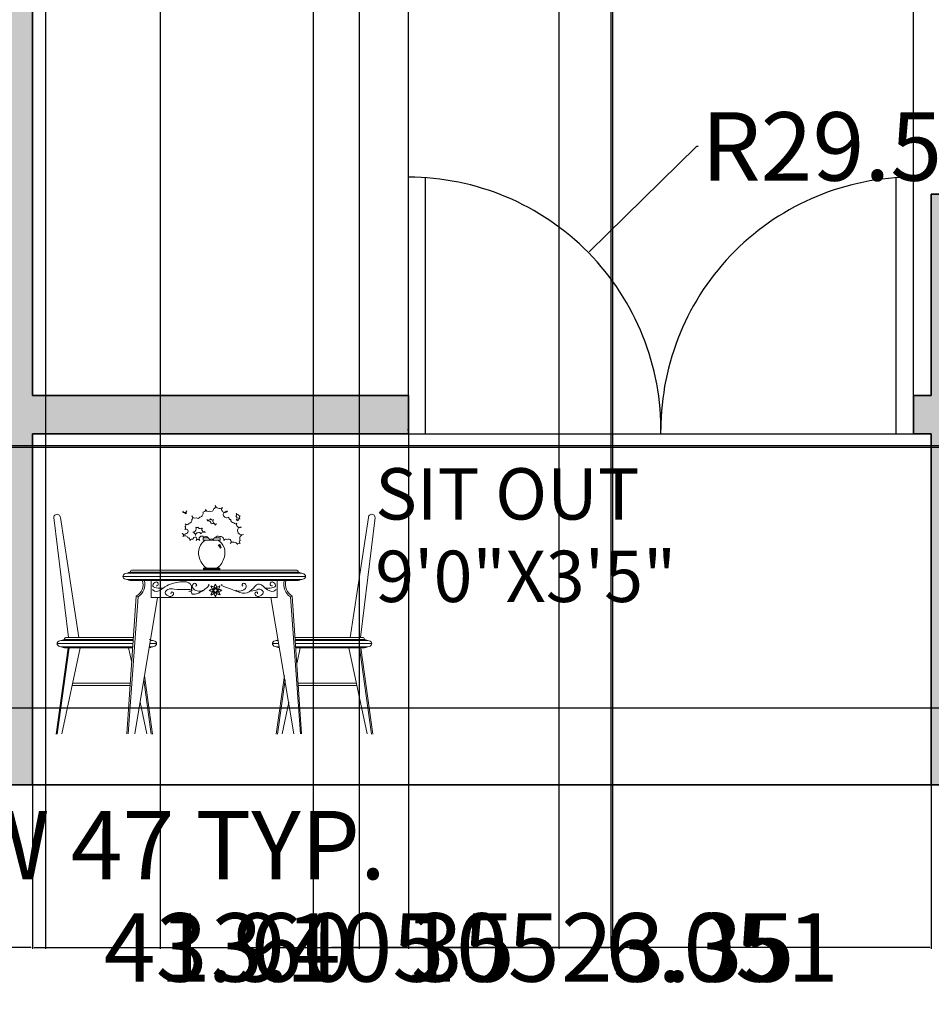
# Model space of a CAD drawing. Units: inches. Extents: x -24 to 368, y -370 to 58.
# Tile 3 of 9: x 130 to 237, y -370 to -255. Entities that reach past the tile are written whole.
import ezdxf

# ---------------------------------------------------------------- set-up
doc = ezdxf.new("R2010")
doc.units = ezdxf.units.IN
doc.header["$MEASUREMENT"] = 0
for name, color, linetype, lineweight in [('A-ANNO-DIMS', 2, 'Continuous', 18), ('A-AREA-IDEN', 7, 'Continuous', 18), ('A-WALL', 7, 'Continuous', 35), ('Furniture', 7, 'Continuous', 15)]:
    doc.layers.add(name, color=color, linetype=linetype, lineweight=lineweight)
doc.layers.add('A-DOOR', color=40, linetype='Continuous', lineweight=25, true_color=0xf8d731)
doc.layers.add('A-WALL-PATT', color=18, linetype='Continuous', lineweight=13, true_color=0x000000)
doc.styles.get("Standard").update_dxf_attribs({"font": 'arial.ttf'})
doc.dimstyles.get("Standard").update_dxf_attribs({"dimtxt": 8, "dimasz": 0.18, "dimexe": 0.18, "dimexo": 0.0625, "dimgap": 0.09, "dimtad": 0, "dimtih": 1, "dimtoh": 1, "dimdec": 4, "dimzin": 0, "dimdsep": 46, "dimlunit": 3, "dimtxsty": 'Standard', "dimcen": 0.09, "dimclre": 5, "dimclrt": 6, "dimadec": 0, "dimazin": 0, "dimtfac": 1, "dimtdec": 4, "dimtofl": 0, "dimtmove": 0, "dimatfit": 3, "dimfxl": 1, "dimtolj": 1, "dimtzin": 0, "dimarcsym": 0})

# ---------------------------------------------------------------- blocks, each defined once
blk = doc.blocks.new('*D15')
at = {"layer": 'A-ANNO-DIMS', "color": 5, "lineweight": -2, "transparency": 16777216}
for p, q in [((37.41, -344.42), (37.41, -351.59)), ((84.41, -344.42), (84.41, -351.59))]:
    blk.add_line(p, q, dxfattribs=at)
at = {"layer": 'A-ANNO-DIMS', "color": 0, "lineweight": -2, "transparency": 16777216}
for p, q in [((37.59, -351.41), (84.23, -351.41)), ((84.41, -351.41), (84.59, -351.41))]:
    blk.add_line(p, q, dxfattribs=at)
at = {"layer": 'A-ANNO-DIMS', "color": 0, "transparency": 16777216}
for points in [[(37.59, -351.38), (37.59, -351.44), (37.41, -351.41)], [(84.23, -351.38), (84.23, -351.44), (84.41, -351.41)]]:
    blk.add_solid(points, dxfattribs=at)
at = {"layer": 'Defpoints', "color": 0, "transparency": 16777216}
for p in [(37.41, -344.36), (84.41, -344.36), (84.41, -351.41)]:
    blk.add_point(p, dxfattribs=at)
at = {"layer": 'A-ANNO-DIMS', "color": 6, "transparency": 16777216, "insert": (130.38, -351.41), "char_height": 8, "attachment_point": 5}
blk.add_mtext('\\A1;WINDOW 47 TYP.', dxfattribs=at)
blk = doc.blocks.new('*D28')
at = {"layer": 'A-ANNO-DIMS', "color": 5, "lineweight": -2, "transparency": 16777216}
for p, q in [((84.41, -344.42), (84.41, -363.55)), ((131.66, -344.42), (131.66, -363.55))]:
    blk.add_line(p, q, dxfattribs=at)
at = {"layer": 'A-ANNO-DIMS', "color": 0, "lineweight": -2, "transparency": 16777216}
for p, q in [((84.59, -363.37), (94.29, -363.37)), ((131.48, -363.37), (121.78, -363.37))]:
    blk.add_line(p, q, dxfattribs=at)
at = {"layer": 'A-ANNO-DIMS', "color": 0, "transparency": 16777216}
for points in [[(84.59, -363.34), (84.59, -363.4), (84.41, -363.37)], [(131.48, -363.34), (131.48, -363.4), (131.66, -363.37)]]:
    blk.add_solid(points, dxfattribs=at)
at = {"layer": 'Defpoints', "color": 0, "transparency": 16777216}
for p in [(84.41, -344.36), (131.66, -344.36), (131.66, -363.37)]:
    blk.add_point(p, dxfattribs=at)
at = {"layer": 'A-ANNO-DIMS', "color": 6, "transparency": 16777216, "insert": (108.03, -363.37), "char_height": 8, "attachment_point": 5}
blk.add_mtext('\\A1;47.26', dxfattribs=at)
blk = doc.blocks.new('*D29')
at = {"layer": 'A-ANNO-DIMS', "color": 5, "lineweight": -2, "transparency": 16777216}
for p, q in [((131.66, -344.42), (131.66, -363.55)), ((236.66, -344.42), (236.66, -363.55))]:
    blk.add_line(p, q, dxfattribs=at)
at = {"layer": 'A-ANNO-DIMS', "color": 0, "lineweight": -2, "transparency": 16777216}
for p, q in [((131.84, -363.37), (175.58, -363.37)), ((236.48, -363.37), (192.74, -363.37))]:
    blk.add_line(p, q, dxfattribs=at)
at = {"layer": 'A-ANNO-DIMS', "color": 0, "transparency": 16777216}
for points in [[(131.84, -363.34), (131.84, -363.4), (131.66, -363.37)], [(236.48, -363.34), (236.48, -363.4), (236.66, -363.37)]]:
    blk.add_solid(points, dxfattribs=at)
at = {"layer": 'Defpoints', "color": 0, "transparency": 16777216}
for p in [(131.66, -344.36), (236.66, -344.36), (236.66, -363.37)]:
    blk.add_point(p, dxfattribs=at)
at = {"layer": 'A-ANNO-DIMS', "color": 6, "transparency": 16777216, "insert": (184.16, -363.37), "char_height": 8, "attachment_point": 5}
blk.add_mtext('\\A1;105', dxfattribs=at)
blk = doc.blocks.new('*D42')
at = {"layer": 'A-ANNO-DIMS', "color": 5, "lineweight": -2, "transparency": 16777216}
for p, q in [((169.81, 24.59), (169.81, -363.55)), ((193.16, 24.58), (193.16, -363.55))]:
    blk.add_line(p, q, dxfattribs=at)
at = {"layer": 'A-ANNO-DIMS', "color": 0, "lineweight": -2, "transparency": 16777216}
for p, q in [((169.99, -363.37), (192.98, -363.37)), ((193.16, -363.37), (193.34, -363.37))]:
    blk.add_line(p, q, dxfattribs=at)
at = {"layer": 'A-ANNO-DIMS', "color": 0, "transparency": 16777216}
for points in [[(169.99, -363.34), (169.99, -363.4), (169.81, -363.37)], [(192.98, -363.34), (192.98, -363.4), (193.16, -363.37)]]:
    blk.add_solid(points, dxfattribs=at)
at = {"layer": 'Defpoints', "color": 0, "transparency": 16777216}
for p in [(169.81, 24.65), (193.16, 24.64), (193.16, -363.37)]:
    blk.add_point(p, dxfattribs=at)
at = {"layer": 'A-ANNO-DIMS', "color": 6, "transparency": 16777216, "insert": (207.03, -363.37), "char_height": 8, "attachment_point": 5}
blk.add_mtext('\\A1;23.35', dxfattribs=at)
blk = doc.blocks.new('*D46')
at = {"layer": 'A-ANNO-DIMS', "color": 5, "lineweight": -2, "transparency": 16777216}
for p, q in [((13.22, -304.91), (341.36, -304.91)), ((13.22, -335.36), (341.36, -335.36))]:
    blk.add_line(p, q, dxfattribs=at)
at = {"layer": 'A-ANNO-DIMS', "color": 0, "lineweight": -2, "transparency": 16777216}
for p, q in [((341.18, -305.09), (341.18, -315.95)), ((341.18, -335.18), (341.18, -324.31))]:
    blk.add_line(p, q, dxfattribs=at)
at = {"layer": 'A-ANNO-DIMS', "color": 0, "transparency": 16777216}
for points in [[(341.15, -305.09), (341.21, -305.09), (341.18, -304.91)], [(341.15, -335.18), (341.21, -335.18), (341.18, -335.36)]]:
    blk.add_solid(points, dxfattribs=at)
at = {"layer": 'Defpoints', "color": 0, "transparency": 16777216}
for p in [(13.16, -304.91), (341.18, -304.91), (13.16, -335.36)]:
    blk.add_point(p, dxfattribs=at)
at = {"layer": 'A-ANNO-DIMS', "color": 6, "transparency": 16777216, "insert": (341.18, -320.13), "char_height": 8, "attachment_point": 5}
blk.add_mtext('\\A1;30.45', dxfattribs=at)
blk = doc.blocks.new('*D51')
at = {"layer": 'A-ANNO-DIMS', "color": 5, "lineweight": -2, "transparency": 16777216}
for p, q in [((175.57, -303.29), (175.57, 52.85)), ((234.57, -303.29), (234.57, 52.85))]:
    blk.add_line(p, q, dxfattribs=at)
at = {"layer": 'A-ANNO-DIMS', "color": 0, "lineweight": -2, "transparency": 16777216}
for p, q in [((175.75, 52.67), (199.24, 52.67)), ((234.39, 52.67), (210.9, 52.67))]:
    blk.add_line(p, q, dxfattribs=at)
at = {"layer": 'A-ANNO-DIMS', "color": 0, "transparency": 16777216}
for points in [[(175.75, 52.7), (175.75, 52.64), (175.57, 52.67)], [(234.39, 52.7), (234.39, 52.64), (234.57, 52.67)]]:
    blk.add_solid(points, dxfattribs=at)
at = {"layer": 'Defpoints', "color": 0, "transparency": 16777216}
for p in [(234.57, 52.67), (175.57, -303.36), (234.57, -303.36)]:
    blk.add_point(p, dxfattribs=at)
at = {"layer": 'A-ANNO-DIMS', "color": 6, "transparency": 16777216, "insert": (205.07, 52.67), "char_height": 8, "attachment_point": 5}
blk.add_mtext('\\A1;59', dxfattribs=at)
blk = doc.blocks.new('*D52')
at = {"layer": 'A-ANNO-DIMS', "color": 5, "lineweight": -2, "transparency": 16777216}
for p, q in [((131.66, -303.42), (131.66, -363.55)), ((175.57, -303.42), (175.57, -363.55))]:
    blk.add_line(p, q, dxfattribs=at)
at = {"layer": 'A-ANNO-DIMS', "color": 0, "lineweight": -2, "transparency": 16777216}
for p, q in [((131.84, -363.37), (140.64, -363.37)), ((175.39, -363.37), (166.59, -363.37))]:
    blk.add_line(p, q, dxfattribs=at)
at = {"layer": 'A-ANNO-DIMS', "color": 0, "transparency": 16777216}
for points in [[(131.84, -363.34), (131.84, -363.4), (131.66, -363.37)], [(175.39, -363.34), (175.39, -363.4), (175.57, -363.37)]]:
    blk.add_solid(points, dxfattribs=at)
at = {"layer": 'Defpoints', "color": 0, "transparency": 16777216}
for p in [(131.66, -303.36), (175.57, -303.36), (175.57, -363.37)]:
    blk.add_point(p, dxfattribs=at)
at = {"layer": 'A-ANNO-DIMS', "color": 6, "transparency": 16777216, "insert": (153.62, -363.37), "char_height": 8, "attachment_point": 5}
blk.add_mtext('\\A1;43.91', dxfattribs=at)
blk = doc.blocks.new('*D56')
at = {"layer": 'A-ANNO-DIMS', "color": 5, "lineweight": -2, "transparency": 16777216}
for p, q in [((164.43, -152.42), (164.43, -363.55)), ((199.43, -152.42), (199.43, -363.55))]:
    blk.add_line(p, q, dxfattribs=at)
at = {"layer": 'A-ANNO-DIMS', "color": 0, "lineweight": -2, "transparency": 16777216}
for p, q in [((164.61, -363.37), (176.08, -363.37)), ((199.25, -363.37), (187.78, -363.37))]:
    blk.add_line(p, q, dxfattribs=at)
at = {"layer": 'A-ANNO-DIMS', "color": 0, "transparency": 16777216}
for points in [[(164.61, -363.34), (164.61, -363.4), (164.43, -363.37)], [(199.25, -363.34), (199.25, -363.4), (199.43, -363.37)]]:
    blk.add_solid(points, dxfattribs=at)
at = {"layer": 'Defpoints', "color": 0, "transparency": 16777216}
for p in [(164.43, -152.36), (199.43, -152.36), (199.43, -363.37)]:
    blk.add_point(p, dxfattribs=at)
at = {"layer": 'A-ANNO-DIMS', "color": 6, "transparency": 16777216, "insert": (181.93, -363.37), "char_height": 8, "attachment_point": 5}
blk.add_mtext('\\A1;35', dxfattribs=at)
blk = doc.blocks.new('*D58')
at = {"layer": 'A-ANNO-DIMS', "color": 5, "lineweight": -2, "transparency": 16777216}
for p, q in [((133.16, -31.92), (133.16, -363.55)), ((146.57, -31.92), (146.57, -363.55))]:
    blk.add_line(p, q, dxfattribs=at)
at = {"layer": 'A-ANNO-DIMS', "color": 0, "lineweight": -2, "transparency": 16777216}
for p, q in [((133.34, -363.37), (146.39, -363.37)), ((146.57, -363.37), (146.75, -363.37))]:
    blk.add_line(p, q, dxfattribs=at)
at = {"layer": 'A-ANNO-DIMS', "color": 0, "transparency": 16777216}
for points in [[(133.34, -363.34), (133.34, -363.4), (133.16, -363.37)], [(146.39, -363.34), (146.39, -363.4), (146.57, -363.37)]]:
    blk.add_solid(points, dxfattribs=at)
at = {"layer": 'Defpoints', "color": 0, "transparency": 16777216}
for p in [(133.16, -31.86), (146.57, -31.86), (146.57, -363.37)]:
    blk.add_point(p, dxfattribs=at)
at = {"layer": 'A-ANNO-DIMS', "color": 6, "transparency": 16777216, "insert": (163.1, -363.37), "char_height": 8, "attachment_point": 5}
blk.add_mtext('\\A1;13.405', dxfattribs=at)
blk = doc.blocks.new('*D60')
at = {"layer": 'A-ANNO-DIMS', "color": 5, "lineweight": -2, "transparency": 16777216}
for p, q in [((133.16, -93.92), (133.16, -363.55)), ((193.16, -95.92), (193.16, -363.55))]:
    blk.add_line(p, q, dxfattribs=at)
at = {"layer": 'A-ANNO-DIMS', "color": 0, "lineweight": -2, "transparency": 16777216}
for p, q in [((133.34, -363.37), (157.33, -363.37)), ((192.98, -363.37), (168.99, -363.37))]:
    blk.add_line(p, q, dxfattribs=at)
at = {"layer": 'A-ANNO-DIMS', "color": 0, "transparency": 16777216}
for points in [[(133.34, -363.34), (133.34, -363.4), (133.16, -363.37)], [(192.98, -363.34), (192.98, -363.4), (193.16, -363.37)]]:
    blk.add_solid(points, dxfattribs=at)
at = {"layer": 'Defpoints', "color": 0, "transparency": 16777216}
for p in [(133.16, -93.86), (193.16, -95.86), (193.16, -363.37)]:
    blk.add_point(p, dxfattribs=at)
at = {"layer": 'A-ANNO-DIMS', "color": 6, "transparency": 16777216, "insert": (163.16, -363.37), "char_height": 8, "attachment_point": 5}
blk.add_mtext('\\A1;60', dxfattribs=at)
blk = doc.blocks.new('*D64')
at = {"layer": 'A-ANNO-DIMS', "color": 5, "lineweight": -2, "transparency": 16777216}
for p, q in [((105.73, -304.73), (341.36, -304.73)), ((106.02, -335.36), (341.36, -335.36))]:
    blk.add_line(p, q, dxfattribs=at)
at = {"layer": 'A-ANNO-DIMS', "color": 0, "lineweight": -2, "transparency": 16777216}
for p, q in [((341.18, -304.91), (341.18, -315.86)), ((341.18, -335.18), (341.18, -324.22))]:
    blk.add_line(p, q, dxfattribs=at)
at = {"layer": 'A-ANNO-DIMS', "color": 0, "transparency": 16777216}
for points in [[(341.15, -304.91), (341.21, -304.91), (341.18, -304.73)], [(341.15, -335.18), (341.21, -335.18), (341.18, -335.36)]]:
    blk.add_solid(points, dxfattribs=at)
at = {"layer": 'Defpoints', "color": 0, "transparency": 16777216}
for p in [(105.67, -304.73), (341.18, -304.73), (105.95, -335.36)]:
    blk.add_point(p, dxfattribs=at)
at = {"layer": 'A-ANNO-DIMS', "color": 6, "transparency": 16777216, "insert": (341.18, -320.04), "char_height": 8, "attachment_point": 5}
blk.add_mtext('\\A1;30.63', dxfattribs=at)
blk = doc.blocks.new('*D65')
at = {"layer": 'A-ANNO-DIMS', "color": 5, "lineweight": -2, "transparency": 16777216}
for p, q in [((105.95, -335.29), (105.95, 52.85)), ((127.16, -335.29), (127.16, 52.85))]:
    blk.add_line(p, q, dxfattribs=at)
at = {"layer": 'A-ANNO-DIMS', "color": 0, "lineweight": -2, "transparency": 16777216}
for p, q in [((106.13, 52.67), (126.98, 52.67)), ((127.16, 52.67), (127.34, 52.67))]:
    blk.add_line(p, q, dxfattribs=at)
at = {"layer": 'A-ANNO-DIMS', "color": 0, "transparency": 16777216}
for points in [[(106.13, 52.7), (106.13, 52.64), (105.95, 52.67)], [(126.98, 52.7), (126.98, 52.64), (127.16, 52.67)]]:
    blk.add_solid(points, dxfattribs=at)
at = {"layer": 'Defpoints', "color": 0, "transparency": 16777216}
for p in [(127.16, 52.67), (105.95, -335.36), (127.16, -335.36)]:
    blk.add_point(p, dxfattribs=at)
at = {"layer": 'A-ANNO-DIMS', "color": 6, "transparency": 16777216, "insert": (140.23, 52.67), "char_height": 8, "attachment_point": 5}
blk.add_mtext('\\A1;21.21', dxfattribs=at)
blk = doc.blocks.new('*D70')
at = {"layer": 'A-ANNO-DIMS', "color": 5, "lineweight": -2, "transparency": 16777216}
for p, q in [((193.16, -95.92), (193.16, -363.55)), ((199.21, -95.92), (199.21, -363.55))]:
    blk.add_line(p, q, dxfattribs=at)
at = {"layer": 'A-ANNO-DIMS', "color": 0, "lineweight": -2, "transparency": 16777216}
for p, q in [((193.34, -363.37), (199.03, -363.37)), ((199.21, -363.37), (199.39, -363.37))]:
    blk.add_line(p, q, dxfattribs=at)
at = {"layer": 'A-ANNO-DIMS', "color": 0, "transparency": 16777216}
for points in [[(193.34, -363.34), (193.34, -363.4), (193.16, -363.37)], [(199.03, -363.34), (199.03, -363.4), (199.21, -363.37)]]:
    blk.add_solid(points, dxfattribs=at)
at = {"layer": 'Defpoints', "color": 0, "transparency": 16777216}
for p in [(193.16, -95.86), (199.21, -95.86), (199.21, -363.37)]:
    blk.add_point(p, dxfattribs=at)
at = {"layer": 'A-ANNO-DIMS', "color": 6, "transparency": 16777216, "insert": (212.23, -363.37), "char_height": 8, "attachment_point": 5}
blk.add_mtext('\\A1;6.051', dxfattribs=at)
blk = doc.blocks.new('*D71')
at = {"layer": 'A-ANNO-DIMS', "color": 0, "lineweight": -2, "transparency": 16777216}
for p, q in [((209.23, -269.76), (196.73, -282.05)), ((209.41, -269.76), (209.23, -269.76))]:
    blk.add_line(p, q, dxfattribs=at)
at = {"layer": 'A-ANNO-DIMS', "color": 5, "lineweight": -2, "transparency": 16777216}
for p, q in [((175.48, -302.86), (175.66, -302.86)), ((175.57, -302.95), (175.57, -302.77))]:
    blk.add_line(p, q, dxfattribs=at)
at = {"layer": 'A-ANNO-DIMS', "color": 0, "transparency": 16777216}
blk.add_solid([(196.71, -282.03), (196.76, -282.07), (196.61, -282.17)], dxfattribs=at)
at = {"layer": 'Defpoints', "color": 0, "transparency": 16777216}
for p in [(196.61, -282.17), (175.57, -302.86)]:
    blk.add_point(p, dxfattribs=at)
at = {"layer": 'A-ANNO-DIMS', "color": 6, "transparency": 16777216, "insert": (229.92, -269.76), "char_height": 8, "attachment_point": 5}
blk.add_mtext('\\A1;R29.504', dxfattribs=at)

msp = doc.modelspace()

# ---------------------------------------------------------------- hatches: boundary and pattern name
at = {"layer": 'A-WALL-PATT'}
h = msp.add_hatch(color=256, dxfattribs=at)
h.dxf.hatch_style = 1
h.paths.add_polyline_path([(13.1621, -93.8573), (80.4499, -93.8573), (80.4499, -89.3573), (13.1621, -89.3573), (13.1621, -61.0987), (4.1621, -61.0987), (4.1621, -149.8573), (13.1621, -149.8573)])
h.paths.add_polyline_path([(146.5668, -27.3573), (133.1621, -27.3573), (133.1621, 10.3323), (133.1272, 10.3313), (133.1621, 24.6427), (139.8141, 24.6427), (139.8141, 33.6427), (95.3329, 33.6427), (95.3329, 24.6427), (128.6621, 24.6427), (128.6621, -89.3573), (127.4499, -89.3573), (127.4499, -93.8573), (133.1621, -93.8573), (133.1621, -31.8573), (146.5668, -31.8573)])
h.paths.add_polyline_path([(197.6621, 24.6427), (236.2134, 24.6427), (236.2134, 33.6427), (169.8141, 33.6427), (169.8141, 24.6427), (193.1621, 24.6427), (193.1621, -27.3573), (181.5668, -27.3573), (181.5668, -31.8573), (193.1621, -31.8573), (193.1621, -95.8573), (199.2127, -95.8573), (199.2127, -91.3573), (197.6621, -91.3573)])
h.paths.add_polyline_path([(322.1621, -52.531), (313.1621, -52.531), (313.1621, -91.3573), (246.2127, -91.3573), (246.2127, -95.8573), (246.6621, -95.8573), (246.6621, -104.9077), (251.1621, -104.9077), (251.1621, -95.8573), (313.1621, -95.8573), (313.1621, -105.6922), (317.6621, -105.6922), (322.1621, -105.6922)])
h.paths.add_polyline_path([(322.1621, -135.6922), (313.1621, -135.6922), (313.1621, -147.8573), (251.1621, -147.8573), (251.1621, -139.9077), (246.6621, -139.9077), (246.6621, -147.8573), (199.43, -147.8573), (199.43, -152.3573), (313.1621, -152.3573), (313.1621, -194.6142), (317.6621, -194.6142), (322.1621, -194.6142)])
h.paths.add_polyline_path([(322.1621, -241.6142), (313.1621, -241.6142), (313.1621, -275.3573), (287.3912, -275.3573), (287.3912, -279.8573), (313.1621, -279.8573), (313.1621, -335.3573), (298.077, -335.3573), (298.077, -344.3573), (322.1621, -344.3573)])
h.paths.add_polyline_path([(263.077, -335.3573), (241.1621, -335.3573), (241.1621, -279.8573), (252.3912, -279.8573), (252.3912, -275.3573), (236.6621, -275.3573), (236.6621, -298.8573), (234.5689, -298.8573), (234.5689, -303.3573), (236.6621, -303.3573), (236.6621, -344.3573), (263.077, -344.3573), (263.077, -339.8573)])
h.paths.add_polyline_path([(175.5689, -298.8573), (131.6621, -298.8573), (131.6621, -152.3573), (164.43, -152.3573), (164.43, -147.8573), (127.1621, -147.8573), (127.1621, -232.8573), (117.1621, -232.8573), (117.1621, -237.3573), (127.1621, -237.3573), (127.1621, -335.3573), (84.4055, -335.3573), (84.4055, -344.3573), (131.6621, -344.3573), (131.6621, -303.3573), (175.5689, -303.3573)])
h.paths.add_polyline_path([(70.1621, -232.8573), (13.1621, -232.8573), (13.1621, -196.8573), (4.1621, -196.8573), (4.1621, -257.9061), (13.1621, -257.9061), (13.1621, -237.3573), (70.1621, -237.3573)])
h.paths.add_polyline_path([(13.1621, -304.9061), (4.1621, -304.9061), (4.1621, -344.3573), (37.4055, -344.3573), (37.4055, -335.3573), (13.1621, -335.3573)])
h.paths.add_polyline_path([(322.1621, 33.6427), (283.2134, 33.6427), (283.2134, 24.6427), (313.1621, 24.6427), (313.1621, 11.9273), (313.4656, 11.629), (313.1621, 11.629), (313.1621, -5.531), (322.1621, -5.531)])
h.paths.add_polyline_path([(48.3329, 33.6427), (4.1621, 33.6427), (4.1621, -14.0987), (13.1621, -14.0987), (13.1621, 24.6427), (48.3329, 24.6427)])

# ---------------------------------------------------------------- linework, layer by layer
at = {"layer": 'A-DOOR'}
for p, q in [((175.5689, -303.3573), (175.5689, -273.3573)), ((177.5689, -303.3573), (177.5689, -273.3573)), ((232.5689, -303.3573), (232.5689, -273.3573)), ((234.5689, -303.3573), (234.5689, -273.3573)), ((175.5689, -298.8573), (175.5689, -303.3573)), ((234.5689, -298.8573), (234.5689, -303.3573)), ((175.5689, -303.3573), (234.5689, -303.3573))]:
    msp.add_line(p, q, dxfattribs=at)
for centre, radius, start, end in [((175.5689, -302.8615), 29.5042, 359.037068, 90), ((234.5689, -302.8531), 29.4958, 90, 180.016185)]:
    msp.add_arc(centre, radius, start, end, dxfattribs=at)
at = {"layer": 'A-WALL'}
for p, q in [((131.6621, -298.8573), (131.6621, -152.3573)), ((236.6621, -275.3573), (236.6621, -298.8573)), ((252.3912, -275.3573), (236.6621, -275.3573)), ((175.5689, -298.8573), (131.6621, -298.8573)), ((236.6621, -298.8573), (234.5689, -298.8573)), ((131.6621, -344.3573), (131.6621, -303.3573)), ((175.5689, -303.3573), (131.6621, -303.3573)), ((236.6621, -303.3573), (234.5689, -303.3573)), ((236.6621, -303.3573), (236.6621, -344.3573)), ((322.1621, -344.3573), (4.1621, -344.3573))]:
    msp.add_line(p, q, dxfattribs=at)
at = {"layer": 'Furniture'}
for p, q in [((135.8503, -327.1311), (134.1515, -313.1372)), ((137.0665, -327.1311), (134.918, -313.1372)), ((168.7647, -327.1311), (170.9132, -313.1372)), ((169.9809, -327.1311), (171.6798, -313.1372)), ((151.5962, -315.7681), (151.5962, -315.4901)), ((152.1996, -315.4901), (151.5962, -315.4901)), ((153.5975, -315.7681), (151.5962, -315.7681)), ((153.5975, -315.4901), (153.0416, -315.4901)), ((153.4992, -316.2761), (153.3679, -316.3866)), ((153.5975, -315.7681), (153.5975, -315.4901)), ((153.7066, -316.5869), (153.5753, -316.6974)), ((162.9698, -319.6366), (142.8068, -319.6366)), ((162.706, -319.5137), (143.0694, -319.5137)), ((162.4915, -319.268), (143.3397, -319.268)), ((151.6287, -319.0514), (151.6287, -319.3097)), ((153.547, -319.0514), (151.6287, -319.0514)), ((153.547, -319.1126), (151.6287, -319.1126)), ((153.547, -319.1839), (151.6287, -319.1839)), ((153.547, -319.0514), (153.547, -319.3097)), ((163.5544, -320.0051), (142.2221, -320.0051)), ((162.9698, -320.3737), (142.8068, -320.3737)), ((162.7065, -320.4966), (143.0694, -320.4966)), ((145.5371, -322.4623), (145.5371, -320.4966)), ((160.2388, -322.4623), (160.2388, -320.4966)), ((152.6166, -321.2765), (152.6067, -321.2468)), ((152.6415, -321.2599), (152.6071, -321.2467)), ((152.6415, -321.2599), (152.617, -321.2764)), ((152.6626, -321.9067), (152.6683, -321.8759)), ((152.6924, -321.9041), (152.663, -321.9066)), ((152.6924, -321.9041), (152.6687, -321.8758)), ((153.0833, -321.5062), (153.089, -321.4754)), ((153.113, -321.5036), (153.0837, -321.5061)), ((153.113, -321.5036), (153.0893, -321.4753)), ((153.1491, -321.7914), (153.1392, -321.7617)), ((153.1681, -321.7725), (153.1396, -321.7616)), ((153.3229, -321.2371), (153.3149, -321.2132)), ((153.3477, -321.2205), (153.3221, -321.2107)), ((153.3477, -321.2205), (153.3233, -321.237)), ((153.3676, -321.8451), (153.3723, -321.8194)), ((153.3973, -321.8424), (153.368, -321.8449)), ((153.3973, -321.8424), (153.377, -321.8181)), ((153.4425, -321.5935), (153.4325, -321.5638)), ((153.4673, -321.5769), (153.4329, -321.5637)), ((153.4673, -321.5769), (153.4429, -321.5934)), ((143.7643, -322.3142), (142.6946, -338.4264)), ((143.9893, -322.4112), (142.8252, -338.4264)), ((146.2743, -322.4623), (143.5955, -338.4264)), ((143.9847, -322.4143), (143.7643, -322.3142)), ((160.2388, -322.4623), (145.5371, -322.4623)), ((152.9505, -322.2262), (152.9526, -322.2148)), ((152.9767, -322.2429), (152.953, -322.2146)), ((152.9767, -322.2429), (152.9604, -322.2443)), ((159.5016, -322.4623), (162.1803, -338.4264)), ((161.7866, -322.4112), (162.9506, -338.4264)), ((161.7911, -322.4143), (162.0115, -322.3142)), ((162.0115, -322.3142), (163.0813, -338.4264)), ((134.531, -327.8682), (143.3956, -327.8682)), ((143.42, -327.4996), (135.1157, -327.4996)), ((143.4282, -327.3768), (135.3794, -327.3768)), ((143.4445, -327.1311), (135.6486, -327.1311)), ((145.3672, -327.8682), (146.1532, -327.8682)), ((145.5686, -327.4996), (145.429, -327.4996)), ((145.9549, -327.8682), (146.1532, -327.8682)), ((159.8763, -327.8682), (159.678, -327.8682)), ((160.4087, -327.8682), (159.678, -327.8682)), ((160.2626, -327.4996), (160.3468, -327.4996)), ((162.3867, -327.1311), (170.1826, -327.1311)), ((162.403, -327.3768), (170.4518, -327.3768)), ((162.4112, -327.4996), (170.7155, -327.4996)), ((171.3002, -327.8682), (162.4357, -327.8682)), ((135.808, -328.3597), (134.4065, -338.4343)), ((135.9595, -328.3597), (134.558, -338.4343)), ((143.3709, -328.2397), (135.0546, -328.2397)), ((137.2121, -328.3597), (135.0878, -338.4264)), ((143.3629, -328.3597), (135.3783, -328.3597)), ((142.8844, -328.3597), (143.2484, -330.0847)), ((145.6297, -328.2397), (145.3048, -328.2397)), ((160.2016, -328.2397), (160.471, -328.2397)), ((162.4603, -328.2397), (170.7766, -328.2397)), ((162.4683, -328.3597), (170.4529, -328.3597)), ((162.9469, -328.3597), (162.5828, -330.0847)), ((168.6191, -328.3597), (170.7434, -338.4264)), ((169.8717, -328.3597), (171.2732, -338.4343)), ((170.0232, -328.3597), (171.4248, -338.4343)), ((143.0881, -332.4987), (136.3387, -332.4987)), ((144.6572, -332.0992), (145.5385, -338.4343)), ((144.7401, -331.6055), (145.6901, -338.4343)), ((161.0912, -331.6055), (160.1412, -338.4343)), ((161.174, -332.0992), (160.2927, -338.4343)), ((162.7431, -332.4987), (169.4925, -332.4987)), ((143.0718, -332.7444), (136.3664, -332.7444)), ((162.7594, -332.7444), (169.5444, -332.7444)), ((144.2215, -334.6959), (145.0087, -338.4264)), ((161.6097, -334.6959), (160.8225, -338.4264))]:
    msp.add_line(p, q, dxfattribs=at)
for centre, radius, start, end in [((152.7358, -311.842), 0.2969, 286.313852, 32.574057), ((153.5211, -311.498), 0.5659, 198.991201, 305.251406), ((134.5347, -313.1313), 0.3833, 359.123141, 180.876859), ((149.3969, -312.3909), 0.1639, 184.864514, 291.124719), ((149.1815, -312.4743), 0.0869, 306.869898, 53.130102), ((149.3101, -312.7314), 0.2026, 5.906141, 112.166346), ((149.4942, -312.3632), 0.1847, 258.055823, 4.316028), ((149.6263, -312.7314), 0.1165, 63.434949, 169.695154), ((149.7826, -312.4882), 0.1737, 126.869898, 233.130102), ((150.5956, -312.8565), 0.3422, 192.907409, 299.167613), ((150.0953, -313.1553), 0.278, 306.869898, 53.130102), ((151.1689, -312.6446), 0.4291, 275.110418, 21.370622), ((151.6067, -312.2207), 0.2702, 261.869898, 8.130102), ((152.1799, -312.1269), 0.3108, 190.304846, 296.565051), ((152.4648, -312.0783), 0.3577, 245.924502, 352.184706), ((154.0144, -312.1825), 0.278, 126.869898, 233.130102), ((154.1395, -312.186), 0.3648, 216.869898, 323.130102), ((154.348, -312.8148), 0.4184, 78.503437, 184.763642), ((154.348, -312.7106), 0.4395, 198.434949, 304.695154), ((155.3173, -312.7592), 0.1942, 296.565051, 42.825256), ((155.2444, -313.204), 0.3146, 313.210089, 59.470294), ((155.6231, -312.6133), 0.1639, 184.864514, 291.124719), ((155.8559, -312.7662), 0.1737, 180, 286.260205), ((155.9288, -313.0233), 0.0936, 105.068488, 211.328693), ((171.2965, -313.1313), 0.3833, 359.123141, 180.876859), ((149.3692, -314.01), 0.1942, 296.565051, 42.825256), ((149.7027, -313.6695), 0.2828, 227.489553, 333.749758), ((149.9529, -313.4715), 0.3231, 270.61606, 16.876265), ((150.9535, -312.9468), 0.2828, 227.489553, 333.749758), ((152.2043, -313.1692), 0.2828, 227.489553, 333.749758), ((152.0027, -313.4784), 0.1013, 337.833654, 84.093859), ((152.1834, -313.8641), 0.3581, 357.776039, 104.036243), ((152.5586, -313.2839), 0.1013, 185.906141, 292.166346), ((152.7393, -314.1351), 0.3245, 21.345787, 127.605991), ((152.708, -313.2943), 0.139, 216.869898, 323.130102), ((152.9547, -313.5583), 0.2258, 126.869898, 233.130102), ((153.0659, -313.6626), 0.2583, 197.216074, 303.476278), ((153.1771, -314.01), 0.1357, 76.675469, 182.935673), ((154.824, -313.1414), 0.2363, 162.897271, 269.157476), ((155.1367, -313.4228), 0.3194, 171.869898, 278.130102), ((155.3833, -313.6313), 0.2285, 208.123735, 314.38394), ((155.5397, -313.5583), 0.1484, 16.313852, 122.574057), ((155.7308, -313.9579), 0.2487, 138.964655, 245.224859), ((155.8072, -313.4367), 0.1484, 106.313852, 212.574057), ((155.835, -313.3464), 0.0869, 36.869898, 143.130102), ((155.9601, -313.1623), 0.1433, 140.906141, 247.166346), ((149.3726, -314.823), 0.278, 216.869898, 323.130102), ((149.0565, -315.2017), 0.2318, 319.864514, 66.124719), ((149.4734, -315.6395), 0.375, 23.4774, 129.737605), ((149.3205, -314.3644), 0.2258, 306.869898, 53.130102), ((149.6158, -314.7084), 0.2285, 28.123735, 134.38394), ((149.5602, -314.7118), 0.2801, 277.125016, 23.385221), ((150.4462, -314.5069), 0.3194, 261.869898, 8.130102), ((150.408, -314.9585), 0.1357, 346.675469, 92.935673), ((150.54, -315.1635), 0.1737, 343.739795, 90), ((150.9604, -315.1635), 0.2583, 84.596209, 190.856413), ((150.8458, -314.1351), 0.1737, 216.869898, 323.130102), ((150.6512, -314.3714), 0.1433, 320.906141, 67.166346), ((151.2175, -314.1733), 0.242, 195.832387, 302.092591), ((151.1133, -315.1114), 0.242, 15.832387, 122.092591), ((151.4295, -314.3158), 0.1042, 216.869898, 323.130102), ((151.6935, -315.1322), 0.3581, 59.703552, 165.963757), ((151.6275, -314.5312), 0.1911, 126.869898, 233.130102), ((151.7456, -314.618), 0.242, 195.832387, 302.092591), ((156.0157, -314.6285), 0.3931, 81.869898, 188.130102), ((155.8697, -314.0448), 0.2801, 209.744881, 316.005086), ((156.1269, -314.6563), 0.5011, 183.17983, 289.440035), ((156.3492, -315.6082), 0.4827, 96.61346, 202.873665), ((149.8139, -315.7264), 0.2363, 342.897271, 89.157476), ((150.2517, -315.8897), 0.2318, 49.864514, 156.124719), ((150.6964, -315.6951), 0.2958, 77.106256, 183.366461), ((150.6165, -315.6013), 0.2432, 306.869898, 53.130102), ((150.9847, -315.9626), 0.278, 36.869898, 143.130102), ((152.7694, -317.2379), 1.721, 121.342885, 197.015329), ((151.353, -315.6013), 0.2432, 126.869898, 233.130102), ((151.4295, -315.5735), 0.278, 36.869898, 143.130102), ((151.8707, -315.8098), 0.4586, 12.246333, 118.506538), ((152.5378, -315.9418), 0.317, 27.407575, 133.66778), ((153.0451, -315.7264), 0.2363, 90.842524, 197.102729), ((153.3161, -315.5874), 0.2912, 54.223922, 160.484127), ((152.4244, -317.2379), 1.721, 342.984671, 58.657115), ((152.8803, -316.9365), 0.735, 18.989745, 48.438613), ((152.9564, -316.8744), 0.735, 18.989745, 48.438613), ((153.5836, -315.7715), 0.4315, 356.76899, 103.029195), ((153.0117, -316.826), 0.735, 18.989745, 48.438613), ((154.2264, -315.8897), 0.2318, 49.864514, 156.124719), ((154.5669, -315.9209), 0.2828, 26.250242, 132.510447), ((154.6433, -315.9453), 0.2318, 293.875281, 40.135486), ((155.1297, -316.5602), 0.5626, 27.989238, 134.249443), ((155.8176, -316.3309), 0.1942, 63.434949, 169.695154), ((156.04, -315.9765), 0.2258, 126.869898, 233.130102), ((153.473, -317.1425), 2.4244, 194.303833, 231.032589), ((151.7208, -317.1425), 2.4244, 308.967411, 345.696167), ((142.4924, -320.0051), 0.2703, 133.570645, 226.429355), ((142.7457, -320.2714), 0.6377, 84.502825, 133.570645), ((143.0677, -319.8521), 0.3384, 89.708291, 140.434352), ((143.3397, -319.5383), 0.2703, 90, 174.784091), ((162.4368, -319.5383), 0.2703, 5.215909, 90), ((162.7089, -319.8521), 0.3384, 39.565648, 90.291709), ((163.0309, -320.2714), 0.6377, 46.429355, 95.497175), ((163.2841, -320.0051), 0.2703, 313.570645, 46.429355), ((142.7457, -319.7389), 0.6377, 226.429355, 275.497175), ((143.0677, -320.1581), 0.3384, 219.565648, 270.291709), ((142.9967, -320.9382), 1.5756, 299.155129, 16.277185), ((142.9967, -320.9382), 1.7762, 303.796641, 13.185856), ((154.0039, -321.6566), 1.1976, 142.485612, 217.514388), ((154.5523, -321.6346), 1.714, 154.818742, 205.181258), ((152.0514, -321.6346), 1.1976, 322.485612, 37.514388), ((151.5029, -321.6566), 1.714, 334.818742, 25.181258), ((162.7792, -320.9382), 1.7762, 166.814144, 236.203359), ((162.7792, -320.9382), 1.5756, 163.722815, 240.844871), ((162.7089, -320.1581), 0.3384, 269.708291, 320.434352), ((163.0309, -319.7389), 0.6377, 264.502825, 313.570645), ((153.0166, -322.6218), 1.1976, 52.485612, 127.514388), ((153.0166, -320.1208), 1.714, 244.818742, 295.181258), ((153.0386, -323.1703), 1.714, 64.818742, 115.181258), ((153.0386, -320.6693), 1.1976, 232.485612, 307.514388), ((154.098, -320.5596), 1.714, 199.818742, 250.181258), ((152.3295, -322.3281), 1.1976, 7.485612, 82.514388), ((154.1135, -322.7159), 1.714, 109.818742, 160.181258), ((152.3451, -320.9475), 1.1976, 277.485612, 352.514388), ((153.7101, -322.3436), 1.1976, 97.485612, 172.514388), ((151.9417, -320.5752), 1.714, 289.818742, 340.181258), ((153.7257, -320.963), 1.1976, 187.485612, 262.514388), ((151.9572, -322.7315), 1.714, 19.818742, 70.181258), ((134.8013, -327.8682), 0.2703, 133.570645, 226.429355), ((135.0546, -328.1344), 0.6377, 84.502825, 133.570645), ((135.3766, -327.7152), 0.3384, 89.708291, 140.434352), ((135.6486, -327.4014), 0.2703, 90, 174.784091), ((145.3077, -327.7152), 0.3384, 39.565648, 90.291709), ((145.6297, -328.1344), 0.6377, 46.429355, 95.497175), ((145.8829, -327.8682), 0.2703, 313.570645, 46.429355), ((159.9483, -327.8682), 0.2703, 133.570645, 226.429355), ((160.2016, -328.1344), 0.6377, 84.502825, 133.570645), ((160.5235, -327.7152), 0.3384, 123.700532, 140.434352), ((170.1826, -327.4014), 0.2703, 5.215909, 90), ((170.4546, -327.7152), 0.3384, 39.565648, 90.291709), ((170.7766, -328.1344), 0.6377, 46.429355, 95.497175), ((171.0299, -327.8682), 0.2703, 313.570645, 46.429355), ((135.0546, -327.602), 0.6377, 226.429355, 275.497175), ((135.3766, -328.0212), 0.3384, 219.565648, 270.291709), ((145.3077, -328.0212), 0.3384, 269.708291, 320.434352), ((145.6297, -327.602), 0.6377, 264.502825, 313.570645), ((160.2016, -327.602), 0.6377, 226.429355, 275.497175), ((160.5235, -328.0212), 0.3384, 219.565648, 264.461782), ((170.4546, -328.0212), 0.3384, 269.708291, 320.434352), ((170.7766, -327.602), 0.6377, 264.502825, 313.570645)]:
    msp.add_arc(centre, radius, start, end, dxfattribs=at)
for points, knots in [([(152.1721, -320.9715), (152.5148, -320.9428), (151.3046, -322.017), (149.9846, -322.3116), (150.5997, -320.3243), (148.0352, -320.6728), (146.9584, -321.3253), (146.1071, -321.9472), (145.7472, -321.6139), (145.6615, -321.5344)], [0, 0, 0, 0, 1.03178829, 2.30706702, 3.06879509, 5.53273575, 6.51138896, 7.57049354, 7.90185408, 7.90185408, 7.90185408, 7.90185408]), ([(146.8549, -321.3689), (146.7013, -321.374), (146.3404, -321.386), (145.5428, -321.2831), (145.8581, -320.6993), (146.3074, -320.5846), (146.4015, -321.1158), (146.1697, -321.1069), (146.0924, -321.104)], [0, 0, 0, 0, 0.49725443, 1.16840045, 1.6574062, 1.92466762, 2.32749044, 2.52912891, 2.52912891, 2.52912891, 2.52912891]), ([(151.4759, -321.6338), (151.7266, -321.797), (150.369, -321.8033), (150.2154, -320.9354), (150.7204, -320.7418), (150.88, -321.0635), (150.754, -321.1192), (150.7135, -321.1371)], [0, 0, 0, 0, 0.89750365, 1.58014669, 1.88576066, 2.13797138, 2.25745142, 2.25745142, 2.25745142, 2.25745142]), ([(153.8305, -320.9715), (153.2296, -320.9212), (155.6018, -321.7901), (156.713, -322.1598), (157.4601, -321.3743), (158.1301, -320.6857), (158.8562, -321.437), (159.6662, -321.9397), (160.0281, -321.6124), (160.1144, -321.5344)], [0, 0, 0, 0, 1.80901962, 3.08429834, 4.28493376, 4.71080628, 5.6894595, 6.74856407, 7.07992461, 7.07992461, 7.07992461, 7.07992461]), ([(155.4714, -321.6338), (155.2207, -321.797), (156.5783, -321.8033), (156.7319, -320.9354), (156.2269, -320.7418), (156.0673, -321.0635), (156.1933, -321.1192), (156.2338, -321.1371)], [0, 0, 0, 0, 0.89750365, 1.58014669, 1.88576066, 2.13797138, 2.25745142, 2.25745142, 2.25745142, 2.25745142]), ([(158.921, -321.3689), (159.0746, -321.374), (159.4355, -321.386), (160.2331, -321.2831), (159.9177, -320.6993), (159.4685, -320.5846), (159.3743, -321.1158), (159.6061, -321.1069), (159.6834, -321.104)], [0, 0, 0, 0, 0.49725443, 1.16840045, 1.6574062, 1.92466762, 2.32749044, 2.52912891, 2.52912891, 2.52912891, 2.52912891]), ([(149.9178, -321.7662), (150.0372, -321.7483), (151.0224, -321.4433), (148.468, -321.6145), (147.5851, -321.3926), (147.0276, -321.8583), (147.4056, -322.301), (147.9445, -322.4844), (148.242, -321.9528), (147.8637, -321.7584), (147.8327, -321.9581), (147.8162, -322.0642)], [0, 0, 0, 0, 0.36194865, 2.42047493, 3.15053252, 3.64302541, 4.00130546, 4.63894482, 5.02654959, 5.24887533, 5.50108583, 5.50108583, 5.50108583, 5.50108583]), ([(157.0294, -321.7662), (156.83, -321.7363), (157.7746, -321.7321), (157.9956, -321.4668), (158.4012, -321.5448), (158.7448, -321.8615), (158.3718, -322.2995), (157.8311, -322.4847), (157.5339, -321.9527), (157.9122, -321.7584), (157.9432, -321.9581), (157.9596, -322.0642)], [0, 0, 0, 0, 0.60491726, 1.12900514, 1.29996463, 1.79245752, 2.15073756, 2.78837692, 3.1759817, 3.39830743, 3.65051793, 3.65051793, 3.65051793, 3.65051793])]:
    msp.add_open_spline(points, degree=3, knots=knots, dxfattribs=at)

# ---------------------------------------------------------------- texts
at = {"layer": 'A-AREA-IDEN'}
for s, p in [('SIT OUT', (171.6953, -313.3646)), ('9\'0"X3\'5"', (171.6953, -323.0031))]:
    msp.add_text(s, height=6, dxfattribs=at).set_placement(p)

# ---------------------------------------------------------------- dimensions: what is measured, and where the dimension line sits
at = {"layer": 'A-ANNO-DIMS'}
for base, p1, p2, override, picture, middle in [((127.1621, 52.6658), (105.953, -335.3573), (127.1621, -335.3573), {"dimdec": 2, "dimlfac": 1, "dimrnd": 0, "dimzin": 0, "dimdsep": 46, "dimlunit": 2}, '*D65', (140.2261, 52.6658)), ((234.5689, 52.6658), (175.5689, -303.3573), (234.5689, -303.3573), {"dimdec": 0, "dimlfac": 1, "dimrnd": 0, "dimzin": 0, "dimdsep": 46, "dimlunit": 2}, '*D51', (205.0689, 52.6658)), ((193.1621, -363.3723), (169.8141, 24.6508), (193.1621, 24.6427), {"dimdec": 2, "dimlfac": 1, "dimrnd": 0, "dimzin": 0, "dimdsep": 46, "dimlunit": 2}, '*D42', (207.0283, -363.3723)), ((146.5668, -363.3723), (133.1621, -31.8573), (146.5668, -31.8573), {"dimdec": 3, "dimlfac": 1, "dimrnd": 0, "dimzin": 0, "dimdsep": 46, "dimlunit": 2}, '*D58', (163.096, -363.3723)), ((193.1621, -363.3723), (133.1621, -93.8573), (193.1621, -95.8573), {"dimdec": 0, "dimlfac": 1, "dimrnd": 0, "dimzin": 0, "dimdsep": 46, "dimlunit": 2}, '*D60', (163.1621, -363.3723)), ((199.2127, -363.3723), (193.1621, -95.8573), (199.2127, -95.8573), {"dimdec": 3, "dimlfac": 1, "dimrnd": 0, "dimzin": 0, "dimdsep": 46, "dimlunit": 2}, '*D70', (212.2304, -363.3723)), ((199.43, -363.3723), (164.43, -152.3573), (199.43, -152.3573), {"dimdec": 0, "dimlfac": 1, "dimrnd": 0, "dimzin": 0, "dimdsep": 46, "dimlunit": 2}, '*D56', (181.93, -363.3723)), ((175.5689, -363.3723), (131.6621, -303.3573), (175.5689, -303.3573), {"dimdec": 2, "dimlfac": 1, "dimrnd": 0, "dimzin": 0, "dimdsep": 46, "dimlunit": 2}, '*D52', (153.6155, -363.3723)), ((131.6621, -363.3723), (84.4055, -344.3573), (131.6621, -344.3573), {"dimdec": 2, "dimlfac": 1, "dimrnd": 0, "dimzin": 0, "dimdsep": 46, "dimlunit": 2}, '*D28', (108.0338, -363.3723)), ((236.6621, -363.3723), (131.6621, -344.3573), (236.6621, -344.3573), {"dimdec": 0, "dimlfac": 1, "dimrnd": 0, "dimzin": 0, "dimdsep": 46, "dimlunit": 2}, '*D29', (184.1621, -363.3723))]:
    dim = msp.add_linear_dim(base=base, p1=p1, p2=p2, dimstyle='Standard', override=override, dxfattribs=at)
    dim.commit()
    dim.dimension.update_dxf_attribs({"geometry": picture, "text_midpoint": middle})
dim = msp.add_radius_dim(center=(175.5689, -302.8615), mpoint=(196.606, -282.175), dimstyle='Standard', override={"dimdec": 3, "dimlfac": 1, "dimrnd": 0, "dimzin": 0, "dimdsep": 46, "dimlunit": 2}, dxfattribs=at)
dim.commit()
dim.dimension.update_dxf_attribs({"geometry": '*D71', "text_midpoint": (229.9158, -269.763), "dimtype": 164})
for base, p1, p2, picture, middle in [((341.1771, -304.9061), (13.1621, -335.3573), (13.1621, -304.9061), '*D46', (341.1771, -320.1317)), ((341.1771, -304.7252), (105.953, -335.3573), (105.6669, -304.7252), '*D64', (341.1771, -320.0412))]:
    dim = msp.add_linear_dim(base=base, p1=p1, p2=p2, angle=90, dimstyle='Standard', override={"dimdec": 2, "dimlfac": 1, "dimrnd": 0, "dimzin": 0, "dimdsep": 46, "dimlunit": 2}, dxfattribs=at)
    dim.commit()
    dim.dimension.update_dxf_attribs({"geometry": picture, "text_midpoint": middle})
dim = msp.add_linear_dim(base=(84.4055, -351.4073), p1=(37.4055, -344.3573), p2=(84.4055, -344.3573), text='WINDOW <> TYP.', dimstyle='Standard', override={"dimdec": 0, "dimlfac": 1, "dimrnd": 0, "dimzin": 0, "dimdsep": 46, "dimlunit": 2}, dxfattribs=at)
dim.commit()
dim.dimension.update_dxf_attribs({"geometry": '*D15', "text_midpoint": (130.3808, -351.4073)})

doc.saveas('drawing.dxf')
